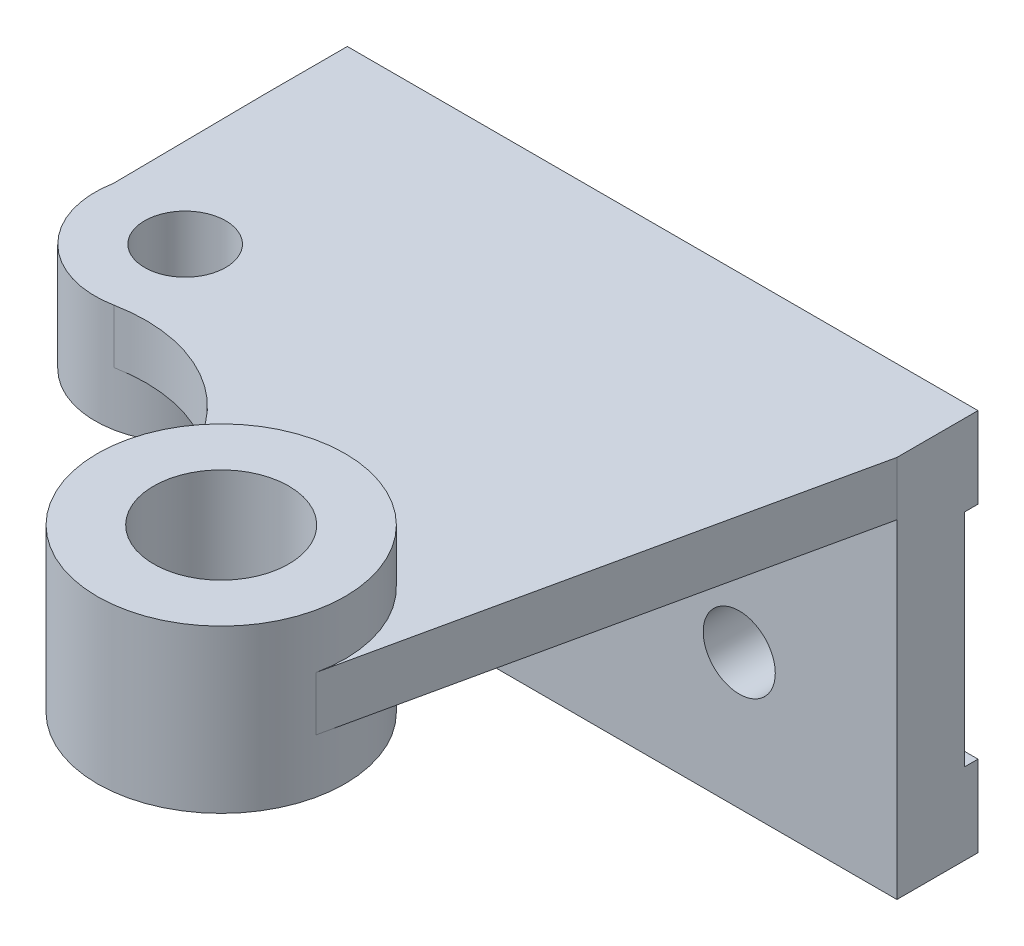
ISO-10303-21;
HEADER;
FILE_DESCRIPTION(('STEP AP214'),'2;1');
FILE_NAME('part.step','',(''),(''),'','','');
FILE_SCHEMA(('AUTOMOTIVE_DESIGN { 1 0 10303 214 1 1 1 1 }'));
ENDSEC;
DATA;
#1=APPLICATION_CONTEXT('core data for automotive mechanical design processes');
#2=APPLICATION_PROTOCOL_DEFINITION('international standard','automotive_design',2000,#1);
#3=PRODUCT_CONTEXT('',#1,'mechanical');
#4=PRODUCT('Part','Part','',(#3));
#5=PRODUCT_RELATED_PRODUCT_CATEGORY('part','',(#4));
#6=PRODUCT_DEFINITION_FORMATION('','',#4);
#7=PRODUCT_DEFINITION_CONTEXT('part definition',#1,'design');
#8=PRODUCT_DEFINITION('design','',#6,#7);
#9=PRODUCT_DEFINITION_SHAPE('','',#8);
#10=(LENGTH_UNIT() NAMED_UNIT(*) SI_UNIT(.MILLI.,.METRE.));
#11=(NAMED_UNIT(*) PLANE_ANGLE_UNIT() SI_UNIT($,.RADIAN.));
#12=(NAMED_UNIT(*) SI_UNIT($,.STERADIAN.) SOLID_ANGLE_UNIT());
#13=UNCERTAINTY_MEASURE_WITH_UNIT(LENGTH_MEASURE(1.E-05),#10,'distance_accuracy_value','');
#14=(GEOMETRIC_REPRESENTATION_CONTEXT(3) GLOBAL_UNCERTAINTY_ASSIGNED_CONTEXT((#13)) GLOBAL_UNIT_ASSIGNED_CONTEXT((#10,
#11,#12)) REPRESENTATION_CONTEXT('',''));
#15=CARTESIAN_POINT('',(0.,0.,0.));
#16=DIRECTION('',(0.,0.,1.));
#17=DIRECTION('',(1.,0.,0.));
#18=AXIS2_PLACEMENT_3D('',#15,#16,#17);
#19=CARTESIAN_POINT('',(90.,-12.,118.));
#20=DIRECTION('',(0.,1.,0.));
#21=DIRECTION('',(0.,0.,1.));
#22=AXIS2_PLACEMENT_3D('',#19,#20,#21);
#23=PLANE('',#22);
#24=CARTESIAN_POINT('',(20.,-12.,56.));
#25=DIRECTION('',(0.,-1.,0.));
#26=DIRECTION('',(0.,0.,-1.));
#27=AXIS2_PLACEMENT_3D('',#24,#25,#26);
#28=CIRCLE('',#27,20.);
#29=CARTESIAN_POINT('',(0.353571949388509,-12.,52.2559560830372));
#30=VERTEX_POINT('',#29);
#31=CARTESIAN_POINT('',(23.863156104059,-12.,75.6233540689575));
#32=VERTEX_POINT('',#31);
#33=EDGE_CURVE('E137',#30,#32,#28,.T.);
#34=ORIENTED_EDGE('',*,*,#33,.F.);
#35=DIRECTION('',(0.0103209239446675,0.,0.999946737846036));
#36=VECTOR('',#35,1.);
#37=CARTESIAN_POINT('',(0.,-12.,18.));
#38=LINE('',#37,#36);
#39=CARTESIAN_POINT('',(0.,-12.,18.));
#40=VERTEX_POINT('',#39);
#41=EDGE_CURVE('E61',#40,#30,#38,.T.);
#42=ORIENTED_EDGE('',*,*,#41,.F.);
#43=DIRECTION('',(-1.,0.,0.));
#44=VECTOR('',#43,1.);
#45=CARTESIAN_POINT('',(0.,-12.,18.));
#46=LINE('',#45,#44);
#47=CARTESIAN_POINT('',(140.,-12.,18.));
#48=VERTEX_POINT('',#47);
#49=EDGE_CURVE('E160',#48,#40,#46,.T.);
#50=ORIENTED_EDGE('',*,*,#49,.F.);
#51=DIRECTION('',(0.213474336033865,0.,-0.97694867206773));
#52=VECTOR('',#51,1.);
#53=CARTESIAN_POINT('',(140.,-12.,18.));
#54=LINE('',#53,#52);
#55=CARTESIAN_POINT('',(116.866088481863,-12.,123.870544240931));
#56=VERTEX_POINT('',#55);
#57=EDGE_CURVE('E164',#56,#48,#54,.T.);
#58=ORIENTED_EDGE('',*,*,#57,.F.);
#59=CARTESIAN_POINT('',(90.,-12.,118.));
#60=DIRECTION('',(0.,-1.,0.));
#61=DIRECTION('',(0.,0.,-1.));
#62=AXIS2_PLACEMENT_3D('',#59,#60,#61);
#63=CIRCLE('',#62,27.5);
#64=CARTESIAN_POINT('',(62.8721271706846,-12.,113.491284467114));
#65=VERTEX_POINT('',#64);
#66=EDGE_CURVE('E325',#65,#56,#63,.T.);
#67=ORIENTED_EDGE('',*,*,#66,.F.);
#68=CARTESIAN_POINT('',(30.2506787778133,-12.,108.069523903741));
#69=DIRECTION('',(0.,-1.,0.));
#70=DIRECTION('',(0.,0.,-1.));
#71=AXIS2_PLACEMENT_3D('',#68,#69,#70);
#72=CIRCLE('',#71,33.0689338028203);
#73=EDGE_CURVE('E145',#32,#65,#72,.T.);
#74=ORIENTED_EDGE('',*,*,#73,.F.);
#75=EDGE_LOOP('',(#34,#42,#50,#58,#67,#74));
#76=FACE_BOUND('',#75,.T.);
#77=ADVANCED_FACE('F44',(#76),#23,.F.);
#78=CARTESIAN_POINT('',(0.,0.,18.));
#79=DIRECTION('',(0.,-1.,0.));
#80=DIRECTION('',(0.,0.,-1.));
#81=AXIS2_PLACEMENT_3D('',#78,#79,#80);
#82=PLANE('',#81);
#83=CARTESIAN_POINT('',(20.,0.,56.));
#84=DIRECTION('',(0.,-1.,0.));
#85=DIRECTION('',(0.,0.,-1.));
#86=AXIS2_PLACEMENT_3D('',#83,#84,#85);
#87=CIRCLE('',#86,9.);
#88=CARTESIAN_POINT('',(20.,0.,47.));
#89=VERTEX_POINT('',#88);
#90=EDGE_CURVE('E309',#89,#89,#87,.T.);
#91=ORIENTED_EDGE('',*,*,#90,.T.);
#92=EDGE_LOOP('',(#91));
#93=FACE_BOUND('',#92,.T.);
#94=CARTESIAN_POINT('',(90.,0.,118.));
#95=DIRECTION('',(0.,1.,0.));
#96=DIRECTION('',(0.,0.,1.));
#97=AXIS2_PLACEMENT_3D('',#94,#95,#96);
#98=CIRCLE('',#97,27.5);
#99=CARTESIAN_POINT('',(116.866088481863,0.,123.870544240931));
#100=VERTEX_POINT('',#99);
#101=CARTESIAN_POINT('',(62.8721271706846,0.,113.491284467114));
#102=VERTEX_POINT('',#101);
#103=EDGE_CURVE('E327',#100,#102,#98,.T.);
#104=ORIENTED_EDGE('',*,*,#103,.F.);
#105=DIRECTION('',(0.213474336033865,0.,-0.97694867206773));
#106=VECTOR('',#105,1.);
#107=CARTESIAN_POINT('',(140.,0.,18.));
#108=LINE('',#107,#106);
#109=CARTESIAN_POINT('',(140.,0.,18.));
#110=VERTEX_POINT('',#109);
#111=EDGE_CURVE('E340',#100,#110,#108,.T.);
#112=ORIENTED_EDGE('',*,*,#111,.T.);
#113=DIRECTION('',(0.,0.,-1.));
#114=VECTOR('',#113,1.);
#115=CARTESIAN_POINT('',(140.,0.,18.));
#116=LINE('',#115,#114);
#117=CARTESIAN_POINT('',(140.,0.,0.));
#118=VERTEX_POINT('',#117);
#119=EDGE_CURVE('E227',#110,#118,#116,.T.);
#120=ORIENTED_EDGE('',*,*,#119,.T.);
#121=DIRECTION('',(-1.,0.,0.));
#122=VECTOR('',#121,1.);
#123=CARTESIAN_POINT('',(0.,0.,0.));
#124=LINE('',#123,#122);
#125=CARTESIAN_POINT('',(0.,0.,0.));
#126=VERTEX_POINT('',#125);
#127=EDGE_CURVE('E221',#118,#126,#124,.T.);
#128=ORIENTED_EDGE('',*,*,#127,.T.);
#129=DIRECTION('',(0.,0.,-1.));
#130=VECTOR('',#129,1.);
#131=CARTESIAN_POINT('',(0.,0.,18.));
#132=LINE('',#131,#130);
#133=CARTESIAN_POINT('',(0.,0.,18.));
#134=VERTEX_POINT('',#133);
#135=EDGE_CURVE('E215',#134,#126,#132,.T.);
#136=ORIENTED_EDGE('',*,*,#135,.F.);
#137=DIRECTION('',(0.0103209239446675,0.,0.999946737846036));
#138=VECTOR('',#137,1.);
#139=CARTESIAN_POINT('',(0.,0.,18.));
#140=LINE('',#139,#138);
#141=CARTESIAN_POINT('',(0.353571949388502,0.,52.2559560830372));
#142=VERTEX_POINT('',#141);
#143=EDGE_CURVE('E337',#134,#142,#140,.T.);
#144=ORIENTED_EDGE('',*,*,#143,.T.);
#145=CARTESIAN_POINT('',(20.,0.,56.));
#146=DIRECTION('',(0.,1.,0.));
#147=DIRECTION('',(0.,0.,1.));
#148=AXIS2_PLACEMENT_3D('',#145,#146,#147);
#149=CIRCLE('',#148,20.);
#150=CARTESIAN_POINT('',(23.863156104059,0.,75.6233540689575));
#151=VERTEX_POINT('',#150);
#152=EDGE_CURVE('E161',#142,#151,#149,.T.);
#153=ORIENTED_EDGE('',*,*,#152,.T.);
#154=CARTESIAN_POINT('',(30.2506787778133,0.,108.069523903741));
#155=DIRECTION('',(0.,-1.,0.));
#156=DIRECTION('',(0.,0.,-1.));
#157=AXIS2_PLACEMENT_3D('',#154,#155,#156);
#158=CIRCLE('',#157,33.0689338028203);
#159=EDGE_CURVE('E344',#151,#102,#158,.T.);
#160=ORIENTED_EDGE('',*,*,#159,.T.);
#161=EDGE_LOOP('',(#104,#112,#120,#128,#136,#144,#153,#160));
#162=FACE_BOUND('',#161,.T.);
#163=ADVANCED_FACE('F260',(#93,#162),#82,.F.);
#164=CARTESIAN_POINT('',(0.,0.,0.));
#165=DIRECTION('',(0.,0.,-1.));
#166=DIRECTION('',(-1.,0.,0.));
#167=AXIS2_PLACEMENT_3D('',#164,#165,#166);
#168=PLANE('',#167);
#169=DIRECTION('',(-1.,0.,0.));
#170=VECTOR('',#169,1.);
#171=CARTESIAN_POINT('',(140.,-67.,0.));
#172=LINE('',#171,#170);
#173=CARTESIAN_POINT('',(140.,-67.,0.));
#174=VERTEX_POINT('',#173);
#175=CARTESIAN_POINT('',(0.,-67.,0.));
#176=VERTEX_POINT('',#175);
#177=EDGE_CURVE('E203',#174,#176,#172,.T.);
#178=ORIENTED_EDGE('',*,*,#177,.F.);
#179=DIRECTION('',(0.,1.,0.));
#180=VECTOR('',#179,1.);
#181=CARTESIAN_POINT('',(140.,0.,0.));
#182=LINE('',#181,#180);
#183=CARTESIAN_POINT('',(140.,-85.,0.));
#184=VERTEX_POINT('',#183);
#185=EDGE_CURVE('E216',#184,#174,#182,.T.);
#186=ORIENTED_EDGE('',*,*,#185,.F.);
#187=DIRECTION('',(1.,0.,0.));
#188=VECTOR('',#187,1.);
#189=CARTESIAN_POINT('',(140.,-85.,0.));
#190=LINE('',#189,#188);
#191=CARTESIAN_POINT('',(0.,-85.,0.));
#192=VERTEX_POINT('',#191);
#193=EDGE_CURVE('E219',#192,#184,#190,.T.);
#194=ORIENTED_EDGE('',*,*,#193,.F.);
#195=DIRECTION('',(0.,-1.,0.));
#196=VECTOR('',#195,1.);
#197=CARTESIAN_POINT('',(0.,-85.,0.));
#198=LINE('',#197,#196);
#199=EDGE_CURVE('E196',#176,#192,#198,.T.);
#200=ORIENTED_EDGE('',*,*,#199,.F.);
#201=EDGE_LOOP('',(#178,#186,#194,#200));
#202=FACE_BOUND('',#201,.T.);
#203=ADVANCED_FACE('F261',(#202),#168,.T.);
#204=CARTESIAN_POINT('',(0.,-85.,18.));
#205=DIRECTION('',(1.,0.,0.));
#206=DIRECTION('',(0.,0.,-1.));
#207=AXIS2_PLACEMENT_3D('',#204,#205,#206);
#208=PLANE('',#207);
#209=DIRECTION('',(0.,1.,0.));
#210=VECTOR('',#209,1.);
#211=CARTESIAN_POINT('',(0.,-18.,3.));
#212=LINE('',#211,#210);
#213=CARTESIAN_POINT('',(0.,-67.,3.));
#214=VERTEX_POINT('',#213);
#215=CARTESIAN_POINT('',(0.,-18.,3.));
#216=VERTEX_POINT('',#215);
#217=EDGE_CURVE('E191',#214,#216,#212,.T.);
#218=ORIENTED_EDGE('',*,*,#217,.F.);
#219=DIRECTION('',(0.,0.,1.));
#220=VECTOR('',#219,1.);
#221=CARTESIAN_POINT('',(0.,-67.,3.));
#222=LINE('',#221,#220);
#223=EDGE_CURVE('E184',#176,#214,#222,.T.);
#224=ORIENTED_EDGE('',*,*,#223,.F.);
#225=ORIENTED_EDGE('',*,*,#199,.T.);
#226=DIRECTION('',(0.,0.,-1.));
#227=VECTOR('',#226,1.);
#228=CARTESIAN_POINT('',(0.,-85.,18.));
#229=LINE('',#228,#227);
#230=CARTESIAN_POINT('',(0.,-85.,18.));
#231=VERTEX_POINT('',#230);
#232=EDGE_CURVE('E11',#231,#192,#229,.T.);
#233=ORIENTED_EDGE('',*,*,#232,.F.);
#234=DIRECTION('',(0.,-1.,0.));
#235=VECTOR('',#234,1.);
#236=CARTESIAN_POINT('',(0.,-85.,18.));
#237=LINE('',#236,#235);
#238=EDGE_CURVE('E206',#40,#231,#237,.T.);
#239=ORIENTED_EDGE('',*,*,#238,.F.);
#240=EDGE_CURVE('E151',#134,#40,#237,.T.);
#241=ORIENTED_EDGE('',*,*,#240,.F.);
#242=ORIENTED_EDGE('',*,*,#135,.T.);
#243=CARTESIAN_POINT('',(0.,-18.,0.));
#244=VERTEX_POINT('',#243);
#245=EDGE_CURVE('E213',#126,#244,#198,.T.);
#246=ORIENTED_EDGE('',*,*,#245,.T.);
#247=DIRECTION('',(0.,0.,-1.));
#248=VECTOR('',#247,1.);
#249=CARTESIAN_POINT('',(0.,-18.,3.));
#250=LINE('',#249,#248);
#251=EDGE_CURVE('E66',#216,#244,#250,.T.);
#252=ORIENTED_EDGE('',*,*,#251,.F.);
#253=EDGE_LOOP('',(#218,#224,#225,#233,#239,#241,#242,#246,#252));
#254=FACE_BOUND('',#253,.T.);
#255=ADVANCED_FACE('F50',(#254),#208,.F.);
#256=CARTESIAN_POINT('',(140.,-85.,18.));
#257=DIRECTION('',(0.,1.,0.));
#258=DIRECTION('',(0.,0.,1.));
#259=AXIS2_PLACEMENT_3D('',#256,#257,#258);
#260=PLANE('',#259);
#261=ORIENTED_EDGE('',*,*,#193,.T.);
#262=DIRECTION('',(0.,0.,-1.));
#263=VECTOR('',#262,1.);
#264=CARTESIAN_POINT('',(140.,-85.,18.));
#265=LINE('',#264,#263);
#266=CARTESIAN_POINT('',(140.,-85.,18.));
#267=VERTEX_POINT('',#266);
#268=EDGE_CURVE('E53',#267,#184,#265,.T.);
#269=ORIENTED_EDGE('',*,*,#268,.F.);
#270=DIRECTION('',(1.,0.,0.));
#271=VECTOR('',#270,1.);
#272=CARTESIAN_POINT('',(140.,-85.,18.));
#273=LINE('',#272,#271);
#274=EDGE_CURVE('E210',#231,#267,#273,.T.);
#275=ORIENTED_EDGE('',*,*,#274,.F.);
#276=ORIENTED_EDGE('',*,*,#232,.T.);
#277=EDGE_LOOP('',(#261,#269,#275,#276));
#278=FACE_BOUND('',#277,.T.);
#279=ADVANCED_FACE('F372',(#278),#260,.F.);
#280=CARTESIAN_POINT('',(140.,0.,18.));
#281=DIRECTION('',(-1.,0.,0.));
#282=DIRECTION('',(0.,0.,1.));
#283=AXIS2_PLACEMENT_3D('',#280,#281,#282);
#284=PLANE('',#283);
#285=ORIENTED_EDGE('',*,*,#185,.T.);
#286=DIRECTION('',(0.,0.,1.));
#287=VECTOR('',#286,1.);
#288=CARTESIAN_POINT('',(140.,-67.,3.));
#289=LINE('',#288,#287);
#290=CARTESIAN_POINT('',(140.,-67.,3.));
#291=VERTEX_POINT('',#290);
#292=EDGE_CURVE('E189',#174,#291,#289,.T.);
#293=ORIENTED_EDGE('',*,*,#292,.T.);
#294=DIRECTION('',(0.,1.,0.));
#295=VECTOR('',#294,1.);
#296=CARTESIAN_POINT('',(140.,-18.,3.));
#297=LINE('',#296,#295);
#298=CARTESIAN_POINT('',(140.,-18.,3.));
#299=VERTEX_POINT('',#298);
#300=EDGE_CURVE('E181',#291,#299,#297,.T.);
#301=ORIENTED_EDGE('',*,*,#300,.T.);
#302=DIRECTION('',(0.,0.,-1.));
#303=VECTOR('',#302,1.);
#304=CARTESIAN_POINT('',(140.,-18.,3.));
#305=LINE('',#304,#303);
#306=CARTESIAN_POINT('',(140.,-18.,0.));
#307=VERTEX_POINT('',#306);
#308=EDGE_CURVE('E183',#299,#307,#305,.T.);
#309=ORIENTED_EDGE('',*,*,#308,.T.);
#310=EDGE_CURVE('E220',#307,#118,#182,.T.);
#311=ORIENTED_EDGE('',*,*,#310,.T.);
#312=ORIENTED_EDGE('',*,*,#119,.F.);
#313=DIRECTION('',(0.,1.,0.));
#314=VECTOR('',#313,1.);
#315=CARTESIAN_POINT('',(140.,-12.,18.));
#316=LINE('',#315,#314);
#317=EDGE_CURVE('E179',#48,#110,#316,.T.);
#318=ORIENTED_EDGE('',*,*,#317,.F.);
#319=DIRECTION('',(0.,1.,0.));
#320=VECTOR('',#319,1.);
#321=CARTESIAN_POINT('',(140.,0.,18.));
#322=LINE('',#321,#320);
#323=EDGE_CURVE('E208',#267,#48,#322,.T.);
#324=ORIENTED_EDGE('',*,*,#323,.F.);
#325=ORIENTED_EDGE('',*,*,#268,.T.);
#326=EDGE_LOOP('',(#285,#293,#301,#309,#311,#312,#318,#324,#325));
#327=FACE_BOUND('',#326,.T.);
#328=ADVANCED_FACE('F357',(#327),#284,.F.);
#329=CARTESIAN_POINT('',(0.,0.,18.));
#330=DIRECTION('',(0.,0.,-1.));
#331=DIRECTION('',(-1.,0.,0.));
#332=AXIS2_PLACEMENT_3D('',#329,#330,#331);
#333=PLANE('',#332);
#334=CARTESIAN_POINT('',(35.,-55.,18.));
#335=DIRECTION('',(0.,0.,1.));
#336=DIRECTION('',(1.,0.,0.));
#337=AXIS2_PLACEMENT_3D('',#334,#335,#336);
#338=CIRCLE('',#337,8.00000000000001);
#339=CARTESIAN_POINT('',(43.,-55.,18.));
#340=VERTEX_POINT('',#339);
#341=EDGE_CURVE('E173',#340,#340,#338,.T.);
#342=ORIENTED_EDGE('',*,*,#341,.F.);
#343=EDGE_LOOP('',(#342));
#344=FACE_BOUND('',#343,.T.);
#345=CARTESIAN_POINT('',(105.,-55.,18.));
#346=DIRECTION('',(0.,0.,1.));
#347=DIRECTION('',(1.,0.,0.));
#348=AXIS2_PLACEMENT_3D('',#345,#346,#347);
#349=CIRCLE('',#348,8.);
#350=CARTESIAN_POINT('',(113.,-55.,18.));
#351=VERTEX_POINT('',#350);
#352=EDGE_CURVE('E180',#351,#351,#349,.T.);
#353=ORIENTED_EDGE('',*,*,#352,.F.);
#354=EDGE_LOOP('',(#353));
#355=FACE_BOUND('',#354,.T.);
#356=ORIENTED_EDGE('',*,*,#323,.T.);
#357=ORIENTED_EDGE('',*,*,#49,.T.);
#358=ORIENTED_EDGE('',*,*,#238,.T.);
#359=ORIENTED_EDGE('',*,*,#274,.T.);
#360=EDGE_LOOP('',(#356,#357,#358,#359));
#361=FACE_BOUND('',#360,.T.);
#362=ADVANCED_FACE('F371',(#344,#355,#361),#333,.F.);
#363=DIRECTION('',(-1.,0.,0.));
#364=VECTOR('',#363,1.);
#365=CARTESIAN_POINT('',(140.,-18.,0.));
#366=LINE('',#365,#364);
#367=EDGE_CURVE('E201',#307,#244,#366,.T.);
#368=ORIENTED_EDGE('',*,*,#367,.T.);
#369=ORIENTED_EDGE('',*,*,#245,.F.);
#370=ORIENTED_EDGE('',*,*,#127,.F.);
#371=ORIENTED_EDGE('',*,*,#310,.F.);
#372=EDGE_LOOP('',(#368,#369,#370,#371));
#373=FACE_BOUND('',#372,.T.);
#374=ADVANCED_FACE('F365',(#373),#168,.T.);
#375=CARTESIAN_POINT('',(140.,-18.,3.));
#376=DIRECTION('',(0.,0.,1.));
#377=DIRECTION('',(1.,0.,0.));
#378=AXIS2_PLACEMENT_3D('',#375,#376,#377);
#379=PLANE('',#378);
#380=CARTESIAN_POINT('',(35.,-55.,2.99999999999999));
#381=DIRECTION('',(0.,0.,1.));
#382=DIRECTION('',(1.,0.,0.));
#383=AXIS2_PLACEMENT_3D('',#380,#381,#382);
#384=CIRCLE('',#383,8.00000000000001);
#385=CARTESIAN_POINT('',(43.,-55.,2.99999999999999));
#386=VERTEX_POINT('',#385);
#387=EDGE_CURVE('E47',#386,#386,#384,.T.);
#388=ORIENTED_EDGE('',*,*,#387,.T.);
#389=EDGE_LOOP('',(#388));
#390=FACE_BOUND('',#389,.T.);
#391=CARTESIAN_POINT('',(105.,-55.,2.99999999999999));
#392=DIRECTION('',(0.,0.,1.));
#393=DIRECTION('',(1.,0.,0.));
#394=AXIS2_PLACEMENT_3D('',#391,#392,#393);
#395=CIRCLE('',#394,8.);
#396=CARTESIAN_POINT('',(113.,-55.,2.99999999999999));
#397=VERTEX_POINT('',#396);
#398=EDGE_CURVE('E176',#397,#397,#395,.T.);
#399=ORIENTED_EDGE('',*,*,#398,.T.);
#400=EDGE_LOOP('',(#399));
#401=FACE_BOUND('',#400,.T.);
#402=ORIENTED_EDGE('',*,*,#217,.T.);
#403=DIRECTION('',(-1.,0.,0.));
#404=VECTOR('',#403,1.);
#405=CARTESIAN_POINT('',(140.,-18.,3.));
#406=LINE('',#405,#404);
#407=EDGE_CURVE('E194',#299,#216,#406,.T.);
#408=ORIENTED_EDGE('',*,*,#407,.F.);
#409=ORIENTED_EDGE('',*,*,#300,.F.);
#410=DIRECTION('',(-1.,0.,0.));
#411=VECTOR('',#410,1.);
#412=CARTESIAN_POINT('',(140.,-67.,3.));
#413=LINE('',#412,#411);
#414=EDGE_CURVE('E197',#291,#214,#413,.T.);
#415=ORIENTED_EDGE('',*,*,#414,.T.);
#416=EDGE_LOOP('',(#402,#408,#409,#415));
#417=FACE_BOUND('',#416,.T.);
#418=ADVANCED_FACE('F240',(#390,#401,#417),#379,.F.);
#419=CARTESIAN_POINT('',(140.,-67.,3.));
#420=DIRECTION('',(0.,-1.,0.));
#421=DIRECTION('',(0.,0.,-1.));
#422=AXIS2_PLACEMENT_3D('',#419,#420,#421);
#423=PLANE('',#422);
#424=ORIENTED_EDGE('',*,*,#223,.T.);
#425=ORIENTED_EDGE('',*,*,#414,.F.);
#426=ORIENTED_EDGE('',*,*,#292,.F.);
#427=ORIENTED_EDGE('',*,*,#177,.T.);
#428=EDGE_LOOP('',(#424,#425,#426,#427));
#429=FACE_BOUND('',#428,.T.);
#430=ADVANCED_FACE('F385',(#429),#423,.F.);
#431=CARTESIAN_POINT('',(140.,-18.,3.));
#432=DIRECTION('',(0.,1.,0.));
#433=DIRECTION('',(0.,0.,1.));
#434=AXIS2_PLACEMENT_3D('',#431,#432,#433);
#435=PLANE('',#434);
#436=ORIENTED_EDGE('',*,*,#251,.T.);
#437=ORIENTED_EDGE('',*,*,#367,.F.);
#438=ORIENTED_EDGE('',*,*,#308,.F.);
#439=ORIENTED_EDGE('',*,*,#407,.T.);
#440=EDGE_LOOP('',(#436,#437,#438,#439));
#441=FACE_BOUND('',#440,.T.);
#442=ADVANCED_FACE('F254',(#441),#435,.F.);
#443=CARTESIAN_POINT('',(105.,-55.,-122.));
#444=DIRECTION('',(0.,0.,1.));
#445=DIRECTION('',(1.,0.,0.));
#446=AXIS2_PLACEMENT_3D('',#443,#444,#445);
#447=CYLINDRICAL_SURFACE('',#446,8.);
#448=ORIENTED_EDGE('',*,*,#352,.T.);
#449=EDGE_LOOP('',(#448));
#450=FACE_BOUND('',#449,.T.);
#451=ORIENTED_EDGE('',*,*,#398,.F.);
#452=EDGE_LOOP('',(#451));
#453=FACE_BOUND('',#452,.T.);
#454=ADVANCED_FACE('F245',(#450,#453),#447,.F.);
#455=CARTESIAN_POINT('',(35.,-55.,-122.));
#456=DIRECTION('',(0.,0.,1.));
#457=DIRECTION('',(1.,0.,0.));
#458=AXIS2_PLACEMENT_3D('',#455,#456,#457);
#459=CYLINDRICAL_SURFACE('',#458,8.00000000000001);
#460=ORIENTED_EDGE('',*,*,#341,.T.);
#461=EDGE_LOOP('',(#460));
#462=FACE_BOUND('',#461,.T.);
#463=ORIENTED_EDGE('',*,*,#387,.F.);
#464=EDGE_LOOP('',(#463));
#465=FACE_BOUND('',#464,.T.);
#466=ADVANCED_FACE('F237',(#462,#465),#459,.F.);
#467=CARTESIAN_POINT('',(140.,-12.,18.));
#468=DIRECTION('',(0.97694867206773,0.,0.213474336033865));
#469=DIRECTION('',(0.213474336033865,0.,-0.97694867206773));
#470=AXIS2_PLACEMENT_3D('',#467,#468,#469);
#471=PLANE('',#470);
#472=ORIENTED_EDGE('',*,*,#111,.F.);
#473=DIRECTION('',(0.,1.,0.));
#474=VECTOR('',#473,1.);
#475=CARTESIAN_POINT('',(116.866088481863,-12.,123.870544240931));
#476=LINE('',#475,#474);
#477=EDGE_CURVE('E349',#56,#100,#476,.T.);
#478=ORIENTED_EDGE('',*,*,#477,.F.);
#479=ORIENTED_EDGE('',*,*,#57,.T.);
#480=ORIENTED_EDGE('',*,*,#317,.T.);
#481=EDGE_LOOP('',(#472,#478,#479,#480));
#482=FACE_BOUND('',#481,.T.);
#483=ADVANCED_FACE('F241',(#482),#471,.T.);
#484=CARTESIAN_POINT('',(30.2506787778133,-12.,108.069523903741));
#485=DIRECTION('',(0.,1.,0.));
#486=DIRECTION('',(0.,0.,1.));
#487=AXIS2_PLACEMENT_3D('',#484,#485,#486);
#488=CYLINDRICAL_SURFACE('',#487,33.0689338028203);
#489=ORIENTED_EDGE('',*,*,#159,.F.);
#490=DIRECTION('',(0.,1.,0.));
#491=VECTOR('',#490,1.);
#492=CARTESIAN_POINT('',(23.863156104059,-12.,75.6233540689575));
#493=LINE('',#492,#491);
#494=EDGE_CURVE('E165',#32,#151,#493,.T.);
#495=ORIENTED_EDGE('',*,*,#494,.F.);
#496=ORIENTED_EDGE('',*,*,#73,.T.);
#497=DIRECTION('',(0.,1.,0.));
#498=VECTOR('',#497,1.);
#499=CARTESIAN_POINT('',(62.8721271706846,-12.,113.491284467114));
#500=LINE('',#499,#498);
#501=EDGE_CURVE('E170',#65,#102,#500,.T.);
#502=ORIENTED_EDGE('',*,*,#501,.T.);
#503=EDGE_LOOP('',(#489,#495,#496,#502));
#504=FACE_BOUND('',#503,.T.);
#505=ADVANCED_FACE('F249',(#504),#488,.F.);
#506=CARTESIAN_POINT('',(0.,-12.,18.));
#507=DIRECTION('',(-0.999946737846036,0.,0.0103209239446675));
#508=DIRECTION('',(0.0103209239446675,0.,0.999946737846036));
#509=AXIS2_PLACEMENT_3D('',#506,#507,#508);
#510=PLANE('',#509);
#511=ORIENTED_EDGE('',*,*,#143,.F.);
#512=ORIENTED_EDGE('',*,*,#240,.T.);
#513=ORIENTED_EDGE('',*,*,#41,.T.);
#514=DIRECTION('',(0.,1.,0.));
#515=VECTOR('',#514,1.);
#516=CARTESIAN_POINT('',(0.353571949388502,-12.,52.2559560830372));
#517=LINE('',#516,#515);
#518=EDGE_CURVE('E154',#30,#142,#517,.T.);
#519=ORIENTED_EDGE('',*,*,#518,.T.);
#520=EDGE_LOOP('',(#511,#512,#513,#519));
#521=FACE_BOUND('',#520,.T.);
#522=ADVANCED_FACE('F153',(#521),#510,.T.);
#523=CARTESIAN_POINT('',(20.,-12.,56.));
#524=DIRECTION('',(0.,1.,0.));
#525=DIRECTION('',(0.,0.,1.));
#526=AXIS2_PLACEMENT_3D('',#523,#524,#525);
#527=CYLINDRICAL_SURFACE('',#526,20.);
#528=ORIENTED_EDGE('',*,*,#518,.F.);
#529=ORIENTED_EDGE('',*,*,#33,.T.);
#530=ORIENTED_EDGE('',*,*,#494,.T.);
#531=ORIENTED_EDGE('',*,*,#152,.F.);
#532=EDGE_LOOP('',(#528,#529,#530,#531));
#533=FACE_BOUND('',#532,.T.);
#534=CARTESIAN_POINT('',(20.,-24.,56.));
#535=DIRECTION('',(0.,-1.,0.));
#536=DIRECTION('',(0.,0.,-1.));
#537=AXIS2_PLACEMENT_3D('',#534,#535,#536);
#538=CIRCLE('',#537,20.);
#539=CARTESIAN_POINT('',(20.,-24.,36.));
#540=VERTEX_POINT('',#539);
#541=EDGE_CURVE('E146',#540,#540,#538,.T.);
#542=ORIENTED_EDGE('',*,*,#541,.F.);
#543=EDGE_LOOP('',(#542));
#544=FACE_BOUND('',#543,.T.);
#545=ADVANCED_FACE('F157',(#533,#544),#527,.T.);
#546=CARTESIAN_POINT('',(90.,-12.,118.));
#547=DIRECTION('',(0.,1.,0.));
#548=DIRECTION('',(0.,0.,1.));
#549=AXIS2_PLACEMENT_3D('',#546,#547,#548);
#550=CYLINDRICAL_SURFACE('',#549,27.5);
#551=ORIENTED_EDGE('',*,*,#501,.F.);
#552=ORIENTED_EDGE('',*,*,#66,.T.);
#553=ORIENTED_EDGE('',*,*,#477,.T.);
#554=ORIENTED_EDGE('',*,*,#103,.T.);
#555=EDGE_LOOP('',(#551,#552,#553,#554));
#556=FACE_BOUND('',#555,.T.);
#557=CARTESIAN_POINT('',(90.,12.,118.));
#558=DIRECTION('',(0.,1.,0.));
#559=DIRECTION('',(0.,0.,1.));
#560=AXIS2_PLACEMENT_3D('',#557,#558,#559);
#561=CIRCLE('',#560,27.5);
#562=CARTESIAN_POINT('',(90.,12.,145.5));
#563=VERTEX_POINT('',#562);
#564=EDGE_CURVE('E326',#563,#563,#561,.T.);
#565=ORIENTED_EDGE('',*,*,#564,.F.);
#566=EDGE_LOOP('',(#565));
#567=FACE_BOUND('',#566,.T.);
#568=CARTESIAN_POINT('',(90.,-24.,118.));
#569=DIRECTION('',(0.,-1.,0.));
#570=DIRECTION('',(0.,0.,-1.));
#571=AXIS2_PLACEMENT_3D('',#568,#569,#570);
#572=CIRCLE('',#571,27.5);
#573=CARTESIAN_POINT('',(90.,-24.,90.5));
#574=VERTEX_POINT('',#573);
#575=EDGE_CURVE('E322',#574,#574,#572,.T.);
#576=ORIENTED_EDGE('',*,*,#575,.F.);
#577=EDGE_LOOP('',(#576));
#578=FACE_BOUND('',#577,.T.);
#579=ADVANCED_FACE('F279',(#556,#567,#578),#550,.T.);
#580=CARTESIAN_POINT('',(90.,12.,118.));
#581=DIRECTION('',(0.,1.,0.));
#582=DIRECTION('',(0.,0.,1.));
#583=AXIS2_PLACEMENT_3D('',#580,#581,#582);
#584=PLANE('',#583);
#585=CARTESIAN_POINT('',(90.,12.,118.));
#586=DIRECTION('',(0.,-1.,0.));
#587=DIRECTION('',(0.,0.,-1.));
#588=AXIS2_PLACEMENT_3D('',#585,#586,#587);
#589=CIRCLE('',#588,15.);
#590=CARTESIAN_POINT('',(90.,12.,103.));
#591=VERTEX_POINT('',#590);
#592=EDGE_CURVE('E150',#591,#591,#589,.T.);
#593=ORIENTED_EDGE('',*,*,#592,.T.);
#594=EDGE_LOOP('',(#593));
#595=FACE_BOUND('',#594,.T.);
#596=ORIENTED_EDGE('',*,*,#564,.T.);
#597=EDGE_LOOP('',(#596));
#598=FACE_BOUND('',#597,.T.);
#599=ADVANCED_FACE('F277',(#595,#598),#584,.T.);
#600=CARTESIAN_POINT('',(90.,-24.,118.));
#601=DIRECTION('',(0.,-1.,0.));
#602=DIRECTION('',(0.,0.,-1.));
#603=AXIS2_PLACEMENT_3D('',#600,#601,#602);
#604=PLANE('',#603);
#605=CARTESIAN_POINT('',(90.,-24.,118.));
#606=DIRECTION('',(0.,-1.,0.));
#607=DIRECTION('',(0.,0.,-1.));
#608=AXIS2_PLACEMENT_3D('',#605,#606,#607);
#609=CIRCLE('',#608,15.);
#610=CARTESIAN_POINT('',(90.,-24.,103.));
#611=VERTEX_POINT('',#610);
#612=EDGE_CURVE('E314',#611,#611,#609,.T.);
#613=ORIENTED_EDGE('',*,*,#612,.F.);
#614=EDGE_LOOP('',(#613));
#615=FACE_BOUND('',#614,.T.);
#616=ORIENTED_EDGE('',*,*,#575,.T.);
#617=EDGE_LOOP('',(#616));
#618=FACE_BOUND('',#617,.T.);
#619=ADVANCED_FACE('F288',(#615,#618),#604,.T.);
#620=CARTESIAN_POINT('',(20.,-24.,56.));
#621=DIRECTION('',(0.,-1.,0.));
#622=DIRECTION('',(0.,0.,-1.));
#623=AXIS2_PLACEMENT_3D('',#620,#621,#622);
#624=PLANE('',#623);
#625=CARTESIAN_POINT('',(20.,-24.,56.));
#626=DIRECTION('',(0.,-1.,0.));
#627=DIRECTION('',(0.,0.,-1.));
#628=AXIS2_PLACEMENT_3D('',#625,#626,#627);
#629=CIRCLE('',#628,9.);
#630=CARTESIAN_POINT('',(20.,-24.,47.));
#631=VERTEX_POINT('',#630);
#632=EDGE_CURVE('E312',#631,#631,#629,.T.);
#633=ORIENTED_EDGE('',*,*,#632,.F.);
#634=EDGE_LOOP('',(#633));
#635=FACE_BOUND('',#634,.T.);
#636=ORIENTED_EDGE('',*,*,#541,.T.);
#637=EDGE_LOOP('',(#636));
#638=FACE_BOUND('',#637,.T.);
#639=ADVANCED_FACE('F291',(#635,#638),#624,.T.);
#640=CARTESIAN_POINT('',(90.,12.,118.));
#641=DIRECTION('',(0.,-1.,0.));
#642=DIRECTION('',(0.,0.,-1.));
#643=AXIS2_PLACEMENT_3D('',#640,#641,#642);
#644=CYLINDRICAL_SURFACE('',#643,15.);
#645=ORIENTED_EDGE('',*,*,#592,.F.);
#646=EDGE_LOOP('',(#645));
#647=FACE_BOUND('',#646,.T.);
#648=ORIENTED_EDGE('',*,*,#612,.T.);
#649=EDGE_LOOP('',(#648));
#650=FACE_BOUND('',#649,.T.);
#651=ADVANCED_FACE('F300',(#647,#650),#644,.F.);
#652=CARTESIAN_POINT('',(20.,0.,56.));
#653=DIRECTION('',(0.,-1.,0.));
#654=DIRECTION('',(0.,0.,-1.));
#655=AXIS2_PLACEMENT_3D('',#652,#653,#654);
#656=CYLINDRICAL_SURFACE('',#655,9.);
#657=ORIENTED_EDGE('',*,*,#90,.F.);
#658=EDGE_LOOP('',(#657));
#659=FACE_BOUND('',#658,.T.);
#660=ORIENTED_EDGE('',*,*,#632,.T.);
#661=EDGE_LOOP('',(#660));
#662=FACE_BOUND('',#661,.T.);
#663=ADVANCED_FACE('F301',(#659,#662),#656,.F.);
#664=CLOSED_SHELL('',(#77,#163,#203,#255,#279,#328,#362,#374,#418,#430,#442,#454,#466,#483,#505,
#522,#545,#579,#599,#619,#639,#651,#663));
#665=MANIFOLD_SOLID_BREP('B2',#664);
#666=ADVANCED_BREP_SHAPE_REPRESENTATION('',(#18,#665),#14);
#667=SHAPE_DEFINITION_REPRESENTATION(#9,#666);
ENDSEC;
END-ISO-10303-21;
